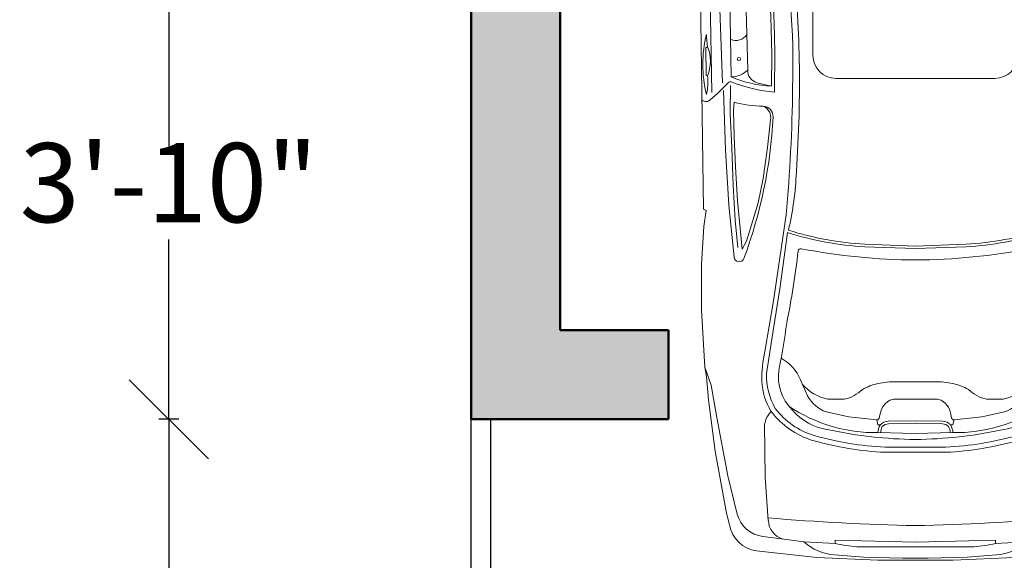
# Model space of a CAD drawing. Units: inches. Extents: x 3121 to 3511, y 1323 to 1998.
# Tile 2 of 10: x 3144 to 3244, y 1402 to 1456. Entities that reach past the tile are written whole.
import ezdxf

# ---------------------------------------------------------------- set-up
doc = ezdxf.new("R2010")
doc.units = ezdxf.units.IN
for name, color, linetype, lineweight in [('0_Equip', 250, 'Continuous', 13), ('A-ANNO-DIMS', 2, 'Continuous', 18), ('A-FLOR', 7, 'Continuous', 25), ('A-WALL', 7, 'Continuous', 50), ('A-WALL-PATT', 3, 'Continuous', 13)]:
    doc.layers.add(name, color=color, linetype=linetype, lineweight=lineweight)
doc.styles.get("Standard").update_dxf_attribs({"font": 'arial.ttf'})
doc.dimstyles.new('ISO-25', dxfattribs={"dimtxt": 8, "dimasz": 8, "dimexe": 1, "dimexo": 1, "dimtad": 0, "dimtih": 1, "dimtoh": 1, "dimlunit": 3, "dimtxsty": 'Standard', "dimblk": 'OBLIQUE', "dimcen": 2.5, "dimclrt": 1, "dimadec": 0, "dimazin": 0, "dimtfac": 1, "dimtmove": 0, "dimatfit": 3, "dimfxl": 1, "dimfxlon": 1, "dimarcsym": 0})

# ---------------------------------------------------------------- blocks, each defined once
blk = doc.blocks.new('A$C4C7B54D1')
at = {"layer": '0_Equip', "ltscale": 0.1}
for p, q in [((-0.7257, 2.678), (-0.8531, 2.6707)), ((-0.7257, 2.678), (-0.5983, 2.6707)), ((-1.112, 2.6343), (-1.2037, 2.6168)), ((-1.0138, 2.6343), (-1.1673, 2.6045)), ((-1.0176, 2.6505), (-1.112, 2.6343)), ((-0.8531, 2.6707), (-1.0176, 2.6505)), ((-0.5983, 2.6707), (-0.4338, 2.6505)), ((-0.4376, 2.6343), (-0.284, 2.6045)), ((-0.4338, 2.6505), (-0.3394, 2.6343)), ((-0.3394, 2.6343), (-0.2477, 2.6168)), ((-1.2037, 2.6168), (-1.3142, 2.5898)), ((-1.1673, 2.6045), (-1.2824, 2.5829)), ((-0.8877, 2.6027), (-0.9812, 2.5937)), ((-0.8072, 2.6112), (-0.8877, 2.6027)), ((-0.7257, 2.6157), (-0.8072, 2.6112)), ((-0.7257, 2.6157), (-0.6441, 2.6112)), ((-0.6441, 2.6112), (-0.5636, 2.6027)), ((-0.5636, 2.6027), (-0.4701, 2.5937)), ((-0.284, 2.6045), (-0.1689, 2.5829)), ((-0.2477, 2.6168), (-0.1371, 2.5898)), ((-1.4032, 2.5628), (-1.4801, 2.5318)), ((-1.3789, 2.557), (-1.4667, 2.5181)), ((-1.3142, 2.5898), (-1.4032, 2.5628)), ((-1.2824, 2.5829), (-1.3789, 2.557)), ((-0.1689, 2.5829), (-0.0725, 2.557)), ((-0.1371, 2.5898), (-0.0481, 2.5628)), ((-0.0725, 2.557), (0.0153, 2.5181)), ((-0.0481, 2.5628), (0.0288, 2.5318)), ((-1.4667, 2.5181), (-1.5113, 2.4907)), ((0.0153, 2.5181), (0.06, 2.4907)), ((-1.5113, 2.4907), (-1.5393, 2.4562)), ((-1.1083, 2.5037), (-1.1486, 2.3827)), ((-0.343, 2.5037), (-0.3027, 2.3827)), ((0.06, 2.4907), (0.0879, 2.4562)), ((-1.5353, 2.3701), (-1.5529, 2.308)), ((-1.435, 2.1869), (-1.4221, 2.3511)), ((-1.1486, 2.3827), (-1.1961, 2.1797)), ((-0.3027, 2.3827), (-0.2552, 2.1797)), ((-0.0163, 2.1869), (-0.0293, 2.3511)), ((0.084, 2.3701), (0.1016, 2.308)), ((-1.5529, 2.308), (-1.5677, 2.2486)), ((0.1016, 2.308), (0.1164, 2.2486)), ((-1.5677, 2.2486), (-1.5849, 2.1795)), ((0.1164, 2.2486), (0.1336, 2.1795)), ((-1.597, 2.1976), (-1.615, 2.1169)), ((-1.6012, 2.2082), (-1.597, 2.1976)), ((-1.4537, 1.863), (-1.435, 2.1869)), ((0.0024, 1.863), (-0.0163, 2.1869)), ((0.1499, 2.2082), (0.1457, 2.1976)), ((0.1457, 2.1976), (0.1637, 2.1169)), ((-1.5849, 2.1795), (-1.5997, 2.1304)), ((-1.1961, 2.1797), (-1.2349, 1.9911)), ((-0.2552, 2.1797), (-0.2164, 1.9911)), ((0.1336, 2.1795), (0.1484, 2.1304)), ((-1.615, 2.1169), (-1.6235, 1.8165)), ((-1.5997, 2.1304), (-1.6161, 2.0798)), ((0.1484, 2.1304), (0.1647, 2.0798)), ((0.1637, 2.1169), (0.1722, 1.8165)), ((-1.2349, 1.9911), (-1.2767, 1.8097)), ((-0.2164, 1.9911), (-0.1746, 1.8097)), ((-1.566, 1.8774), (-1.5761, 1.5304)), ((-1.4681, 1.48), (-1.4537, 1.863)), ((0.0168, 1.48), (0.0024, 1.863)), ((0.1147, 1.8774), (0.1247, 1.5304)), ((-1.6235, 1.8165), (-1.6256, 1.5098)), ((-1.2767, 1.8097), (-1.3098, 1.588)), ((-0.1746, 1.8097), (-0.1415, 1.588)), ((0.1722, 1.8165), (0.1743, 1.5098)), ((-1.3098, 1.588), (-1.3443, 1.3187)), ((-0.1415, 1.588), (-0.107, 1.3187)), ((-1.6256, 1.5098), (-1.6129, 1.3846)), ((-1.5761, 1.5304), (-1.5789, 1.1834)), ((0.1247, 1.5304), (0.1276, 1.1834)), ((0.1743, 1.5098), (0.1616, 1.3846)), ((-1.461, 1.1868), (-1.4681, 1.48)), ((-0.955, 1.4459), (-0.955, 1.4827)), ((-0.955, 1.4827), (-0.9321, 1.4827)), ((-0.9321, 1.4827), (-0.9321, 1.4459)), ((-0.5192, 1.4827), (-0.5192, 1.4459)), ((-0.4964, 1.4827), (-0.5192, 1.4827)), ((-0.4964, 1.4459), (-0.4964, 1.4827)), ((0.0097, 1.1868), (0.0168, 1.48)), ((-0.9321, 1.4459), (-0.955, 1.4459)), ((-0.8614, 1.4242), (-0.8603, 1.382)), ((-0.6135, 1.4258), (-0.6012, 1.3814)), ((-0.5809, 1.3459), (-0.5793, 1.4233)), ((-0.5192, 1.4459), (-0.4964, 1.4459)), ((-1.6193, 1.3782), (-1.6252, 0.9375)), ((-1.6129, 1.3846), (-1.6193, 1.3782)), ((-0.8878, 1.3764), (-1.0456, 1.313)), ((-0.7861, 1.3973), (-0.8878, 1.3764)), ((0.1616, 1.3846), (0.1679, 1.3782)), ((0.1679, 1.3782), (0.1739, 0.9375)), ((-0.8835, 1.3269), (-0.7975, 1.3408)), ((-1.0456, 1.313), (-1.4462, 1.1776)), ((-1.0263, 1.2883), (-0.9361, 1.3119)), ((-0.9361, 1.3119), (-0.8835, 1.3269)), ((-1.2207, 1.2292), (-1.0263, 1.2883)), ((-1.4366, 1.1604), (-1.2207, 1.2292)), ((-1.3162, 1.2215), (-1.3088, 1.2011)), ((-1.0667, 1.22), (-1.1723, 1.1976)), ((-0.3847, 1.22), (-0.279, 1.1976)), ((-1.4565, 1.1447), (-1.461, 1.1868)), ((-1.4462, 1.1776), (-1.4366, 1.1604)), ((-1.1723, 1.1976), (-1.2762, 1.1716)), ((-0.7257, 1.1776), (-0.8858, 1.1725)), ((-0.7257, 1.1776), (-0.5655, 1.1725)), ((-0.279, 1.1976), (-0.1751, 1.1716)), ((0.0052, 1.1447), (0.0097, 1.1868)), ((-1.5793, 1.1562), (-1.5793, 0.9761)), ((-1.5552, 1.139), (-1.5552, 0.9693)), ((-1.4503, 1.1151), (-1.4565, 1.1447)), ((-1.3515, 1.142), (-1.3703, 1.1286)), ((-1.2762, 1.1716), (-1.3515, 1.142)), ((-0.1751, 1.1716), (-0.0999, 1.142)), ((-0.0999, 1.142), (-0.0811, 1.1286)), ((-0.0011, 1.1151), (0.0052, 1.1447)), ((0.1038, 1.139), (0.1038, 0.9693)), ((0.128, 1.1562), (0.128, 0.9761)), ((-1.444, 1.0892), (-1.4503, 1.1151)), ((-1.39, 1.0981), (-1.3927, 1.0739)), ((-1.3828, 1.1133), (-1.39, 1.0981)), ((-1.3703, 1.1286), (-1.3828, 1.1133)), ((-0.0811, 1.1286), (-0.0685, 1.1133)), ((-0.0685, 1.1133), (-0.0614, 1.0981)), ((-0.0614, 1.0981), (-0.0587, 1.0739)), ((-0.0073, 1.0892), (-0.0011, 1.1151)), ((-1.4368, 1.0623), (-1.444, 1.0892)), ((-1.4243, 1.0229), (-1.4368, 1.0623)), ((-1.3927, 1.0739), (-1.3918, 1.0533)), ((-1.3918, 1.0533), (-1.3867, 1.0211)), ((-0.0596, 1.0533), (-0.0646, 1.0211)), ((-0.0587, 1.0739), (-0.0596, 1.0533)), ((-0.027, 1.0229), (-0.0145, 1.0623)), ((-0.0145, 1.0623), (-0.0073, 1.0892)), ((-1.4064, 0.961), (-1.4243, 1.0229)), ((-1.3867, 1.0211), (-1.3374, 0.8446)), ((-0.0646, 1.0211), (-0.1139, 0.8446)), ((-0.0449, 0.961), (-0.027, 1.0229)), ((-1.5149, 1.011), (-1.4844, 0.9277)), ((0.0635, 1.011), (0.0331, 0.9277)), ((-1.6252, 0.9375), (-1.6745, 0.908)), ((-1.6252, 0.9375), (-1.5546, 0.9696)), ((-1.3759, 0.8562), (-1.4064, 0.961)), ((-0.0754, 0.8562), (-0.0449, 0.961)), ((0.1739, 0.9375), (0.1032, 0.9696)), ((0.1739, 0.9375), (0.2232, 0.908)), ((-1.6745, 0.908), (-1.7088, 0.8764)), ((-1.508, 0.8914), (-1.5321, 0.8786)), ((-1.4844, 0.9277), (-1.4486, 0.8345)), ((0.0331, 0.9277), (-0.0028, 0.8345)), ((0.0566, 0.8914), (0.0807, 0.8786)), ((0.2232, 0.908), (0.2574, 0.8764)), ((-1.5321, 0.8786), (-1.7381, 0.7945)), ((-1.5253, 0.865), (-1.7329, 0.7802)), ((-1.7088, 0.8764), (-1.728, 0.8432)), ((-1.5273, 0.8512), (-1.7203, 0.7738)), ((-1.4835, -0.0735), (-1.497, 0.863)), ((-1.3401, 0.7406), (-1.3759, 0.8562)), ((-0.1112, 0.7406), (-0.0754, 0.8562)), ((0.0322, -0.0735), (0.0457, 0.863)), ((0.074, 0.865), (0.2816, 0.7802)), ((0.0759, 0.8512), (0.269, 0.7738)), ((0.0807, 0.8786), (0.2867, 0.7945)), ((0.2574, 0.8764), (0.2767, 0.8432)), ((-1.7366, 0.8127), (-1.7377, 0.7934)), ((-1.728, 0.8432), (-1.7366, 0.8127)), ((-1.6171, 0.8152), (-1.5964, -0.6171)), ((-1.5805, 0.8299), (-1.5623, -0.138)), ((-1.5337, 0.8406), (-1.5355, 0.484)), ((-1.4486, 0.8345), (-1.4226, 0.7503)), ((-1.3374, 0.8446), (-1.3097, 0.7577)), ((-0.1139, 0.8446), (-0.1417, 0.7577)), ((-0.0028, 0.8345), (-0.0287, 0.7503)), ((0.0824, 0.8406), (0.0842, 0.484)), ((0.1292, 0.8299), (0.111, -0.138)), ((0.1658, 0.8152), (0.145, -0.6171)), ((0.2767, 0.8432), (0.2853, 0.8127)), ((0.2853, 0.8127), (0.2863, 0.7934)), ((-1.7377, 0.7934), (-1.7327, 0.7794)), ((-1.4352, 0.792), (-1.4152, -0.045)), ((-0.0162, 0.792), (-0.0361, -0.045)), ((0.2863, 0.7934), (0.2813, 0.7794)), ((-1.4226, 0.7503), (-1.4029, 0.6849)), ((-1.315, 0.66), (-1.3401, 0.7406)), ((-1.3097, 0.7577), (-1.2953, 0.7129)), ((-0.7926, 0.7532), (-0.8418, 0.7514)), ((-0.7257, 0.7541), (-0.7926, 0.7532)), ((-0.7257, 0.7541), (-0.6587, 0.7532)), ((-0.6587, 0.7532), (-0.6095, 0.7514)), ((-0.1417, 0.7577), (-0.156, 0.7129)), ((-0.1363, 0.66), (-0.1112, 0.7406)), ((-0.0287, 0.7503), (-0.0484, 0.6849)), ((-1.2953, 0.7129), (-1.2801, 0.6573)), ((-0.156, 0.7129), (-0.1712, 0.6573)), ((-1.4029, 0.6849), (-1.368, 0.5729)), ((-1.2951, 0.5849), (-1.315, 0.66)), ((-1.2801, 0.6573), (-1.2795, 0.6546)), ((-0.9389, 0.6526), (-1.0437, 0.6403)), ((-0.8346, 0.6593), (-0.9389, 0.6526)), ((-0.7257, 0.6582), (-0.8346, 0.6593)), ((-0.7257, 0.6582), (-0.6168, 0.6593)), ((-0.6168, 0.6593), (-0.5124, 0.6526)), ((-0.5124, 0.6526), (-0.4076, 0.6403)), ((-0.1712, 0.6573), (-0.1719, 0.6546)), ((-0.1562, 0.5849), (-0.1363, 0.66)), ((-0.0484, 0.6849), (-0.0834, 0.5729)), ((-1.2021, 0.6133), (-1.2663, 0.5956)), ((-1.1177, 0.6302), (-1.2021, 0.6133)), ((-1.1142, 0.6096), (-1.1973, 0.593)), ((-1.0437, 0.6403), (-1.1177, 0.6302)), ((-1.0411, 0.6196), (-1.1142, 0.6096)), ((-0.937, 0.6317), (-1.0411, 0.6196)), ((-0.834, 0.6384), (-0.937, 0.6317)), ((-0.7257, 0.6373), (-0.834, 0.6384)), ((-0.7257, 0.6373), (-0.6173, 0.6384)), ((-0.6173, 0.6384), (-0.5143, 0.6317)), ((-0.5143, 0.6317), (-0.4102, 0.6196)), ((-0.4102, 0.6196), (-0.3371, 0.6096)), ((-0.4076, 0.6403), (-0.3337, 0.6302)), ((-0.3371, 0.6096), (-0.2541, 0.593)), ((-0.3337, 0.6302), (-0.2492, 0.6133)), ((-0.2492, 0.6133), (-0.185, 0.5956)), ((-1.368, 0.5729), (-1.3527, 0.5066)), ((-1.2663, 0.5956), (-1.2951, 0.5849)), ((-1.2879, 0.5653), (-1.2951, 0.5849)), ((-1.2599, 0.5757), (-1.2879, 0.5653)), ((-1.1973, 0.593), (-1.2599, 0.5757)), ((-0.2541, 0.593), (-0.1914, 0.5757)), ((-0.1914, 0.5757), (-0.1635, 0.5653)), ((-0.185, 0.5956), (-0.1562, 0.5849)), ((-0.1635, 0.5653), (-0.1562, 0.5849)), ((-0.0834, 0.5729), (-0.0986, 0.5066)), ((-1.3527, 0.5066), (-1.3411, 0.4394)), ((-0.0986, 0.5066), (-0.1102, 0.4394)), ((-1.5355, 0.484), (-1.5292, 0.2045)), ((0.0842, 0.484), (0.0779, 0.2045)), ((-1.3411, 0.4394), (-1.3321, 0.3749)), ((-0.7257, 0.4085), (-1.0528, 0.4085)), ((-0.7257, 0.4085), (-0.3986, 0.4085)), ((-0.1102, 0.4394), (-0.1192, 0.3749)), ((-1.3321, 0.3749), (-1.3286, 0.3301)), ((-0.1192, 0.3749), (-0.1228, 0.3301)), ((-1.3286, 0.3301), (-1.3204, 0.1751)), ((-1.3178, 0.3418), (-1.31, 0.2426)), ((-0.1335, 0.3418), (-0.1413, 0.2426)), ((-0.1228, 0.3301), (-0.1309, 0.1751)), ((-1.1468, 0.3145), (-1.1468, 0.0145)), ((-0.3045, 0.3145), (-0.3045, 0.0145)), ((-1.5292, 0.2045), (-1.5185, -0.0974)), ((-1.31, 0.2426), (-1.306, 0.1454)), ((-0.1413, 0.2426), (-0.1454, 0.1454)), ((0.0779, 0.2045), (0.0672, -0.0974)), ((-1.3204, 0.1751), (-1.3164, 0.0193)), ((-0.1309, 0.1751), (-0.1349, 0.0193)), ((-1.306, 0.1454), (-1.3036, 0.0305)), ((-0.1454, 0.1454), (-0.1478, 0.0305)), ((-1.5798, 0.0505), (-1.5879, 0.0456)), ((-1.5879, 0.0456), (-1.5863, -0.0676)), ((0.1285, 0.0505), (0.1365, 0.0456)), ((0.1365, 0.0456), (0.1349, -0.0676)), ((-1.3164, 0.0193), (-1.3178, -0.1112)), ((-1.3036, 0.0305), (-1.3044, -0.1358)), ((-0.1478, 0.0305), (-0.147, -0.1358)), ((-0.1349, 0.0193), (-0.1335, -0.1112)), ((-1.5863, -0.0676), (-1.5806, -0.0692)), ((-0.7257, -0.0796), (-1.0528, -0.0796)), ((-0.7257, -0.0796), (-0.3986, -0.0796)), ((0.1349, -0.0676), (0.1293, -0.0692)), ((-1.4948, -0.0965), (-1.5413, -0.143)), ((-1.4857, -0.1082), (-1.4866, -0.2223)), ((-1.3774, -0.0972), (-1.3178, -0.1112)), ((-0.0739, -0.0972), (-0.1335, -0.1112)), ((0.0344, -0.1082), (0.0352, -0.2223)), ((0.0435, -0.0965), (0.0899, -0.143)), ((-1.5413, -0.143), (-1.5686, -0.1663)), ((-1.5147, -0.1299), (-1.5058, -0.3725)), ((0.0633, -0.1299), (0.0545, -0.3725)), ((0.0899, -0.143), (0.1172, -0.1663)), ((-1.4713, -0.1773), (-1.4737, -0.2127)), ((0.02, -0.1773), (0.0224, -0.2127)), ((-1.4866, -0.2223), (-1.4809, -0.3653)), ((-1.4737, -0.2127), (-1.4705, -0.3187)), ((0.0224, -0.2127), (0.0192, -0.3187)), ((0.0352, -0.2223), (0.0296, -0.3653)), ((-1.3211, -0.2496), (-1.3332, -0.3629)), ((-0.1302, -0.2496), (-0.1182, -0.3629)), ((-1.4705, -0.3187), (-1.4649, -0.4424)), ((0.0192, -0.3187), (0.0135, -0.4424)), ((-1.3332, -0.3629), (-1.3516, -0.4906)), ((-0.1182, -0.3629), (-0.0997, -0.4906)), ((-1.5058, -0.3725), (-1.4922, -0.6007)), ((-1.4809, -0.3653), (-1.4745, -0.5203)), ((0.0296, -0.3653), (0.0232, -0.5203)), ((0.0545, -0.3725), (0.0408, -0.6007)), ((-1.4649, -0.4424), (-1.4576, -0.5822)), ((0.0135, -0.4424), (0.0063, -0.5822)), ((-1.4745, -0.5203), (-1.4665, -0.6617)), ((-1.3516, -0.4906), (-1.3725, -0.5902)), ((-0.0997, -0.4906), (-0.0788, -0.5902)), ((0.0232, -0.5203), (0.0151, -0.6617)), ((-1.4922, -0.6007), (-1.4712, -0.814)), ((-1.4576, -0.5822), (-1.4384, -0.7806)), ((-1.3725, -0.5902), (-1.3942, -0.6641)), ((-0.0788, -0.5902), (-0.0571, -0.6641)), ((0.0063, -0.5822), (-0.013, -0.7806)), ((0.0408, -0.6007), (0.0198, -0.814)), ((-1.5964, -0.6171), (-1.5863, -0.6228)), ((-1.5863, -0.6228), (-1.5949, -0.6885)), ((-1.3094, -0.9936), (-1.2569, -0.6398)), ((-0.1419, -0.9936), (-0.1944, -0.6398)), ((0.145, -0.6171), (0.1349, -0.6228)), ((0.1349, -0.6228), (0.1436, -0.6885)), ((-1.4665, -0.6617), (-1.4552, -0.7742)), ((-1.3942, -0.6641), (-1.4199, -0.7485)), ((-0.0571, -0.6641), (-0.0314, -0.7485)), ((0.0151, -0.6617), (0.0039, -0.7742)), ((-1.5949, -0.6885), (-1.605, -0.843)), ((-1.2616, -0.7846), (-1.2511, -0.7134)), ((-0.1898, -0.7846), (-0.2003, -0.7134)), ((0.1436, -0.6885), (0.1537, -0.843)), ((-1.4199, -0.7485), (-1.4384, -0.7806)), ((-0.9331, -0.7613), (-0.7253, -0.7683)), ((-0.5182, -0.7613), (-0.726, -0.7683)), ((-0.0314, -0.7485), (-0.013, -0.7806)), ((-1.2826, -0.9445), (-1.2616, -0.7846)), ((-0.9336, -0.7717), (-0.7257, -0.7787)), ((-0.5177, -0.7717), (-0.7257, -0.7787)), ((-0.1688, -0.9445), (-0.1898, -0.7846)), ((-1.605, -0.843), (-1.605, -1.0322)), ((0.1537, -0.843), (0.1537, -1.0322)), ((-1.3094, -1.1068), (-1.2826, -0.9445)), ((-0.1419, -1.1068), (-0.1688, -0.9445)), ((-1.3444, -1.2014), (-1.3094, -0.9936)), ((-0.1069, -1.2014), (-0.1419, -0.9936)), ((-1.605, -1.0322), (-1.592, -1.2661)), ((0.1537, -1.0322), (0.1407, -1.2661)), ((-1.3386, -1.2925), (-1.3094, -1.1068)), ((-0.1127, -1.2925), (-0.1419, -1.1068)), ((-1.565, -1.3405), (-1.592, -1.2661)), ((-1.592, -1.2661), (-1.5848, -1.3051)), ((0.1137, -1.3405), (0.1407, -1.2661)), ((0.1407, -1.2661), (0.1335, -1.3051)), ((-1.5848, -1.3051), (-1.5762, -1.4004)), ((-1.1985, -1.3182), (-1.1694, -1.3835)), ((-0.88, -1.3337), (-0.8328, -1.3271)), ((-0.8328, -1.3271), (-0.7257, -1.3271)), ((-0.6185, -1.3271), (-0.7257, -1.3271)), ((-0.5713, -1.3337), (-0.6185, -1.3271)), ((-0.2528, -1.3182), (-0.282, -1.3835)), ((0.1335, -1.3051), (0.1248, -1.4004)), ((-1.5417, -1.4736), (-1.565, -1.3405)), ((0.0904, -1.4736), (0.1137, -1.3405)), ((-1.5762, -1.4004), (-1.5486, -1.6107)), ((-1.0858, -1.3979), (-1.0181, -1.3979)), ((-0.8488, -1.4158), (-0.8558, -1.4236)), ((-0.8409, -1.4088), (-0.8488, -1.4158)), ((-0.8309, -1.402), (-0.8409, -1.4088)), ((-0.8163, -1.3979), (-0.8309, -1.402)), ((-0.7257, -1.3974), (-0.8163, -1.3979)), ((-0.7257, -1.3974), (-0.635, -1.3979)), ((-0.635, -1.3979), (-0.6204, -1.402)), ((-0.6204, -1.402), (-0.6104, -1.4088)), ((-0.6104, -1.4088), (-0.6025, -1.4158)), ((-0.6025, -1.4158), (-0.5955, -1.4236)), ((-0.3655, -1.3979), (-0.4333, -1.3979)), ((0.1248, -1.4004), (0.0973, -1.6107)), ((-1.0923, -1.4501), (-0.9989, -1.4699)), ((-0.8696, -1.4545), (-0.8731, -1.467)), ((-0.8664, -1.4423), (-0.8696, -1.4545)), ((-0.861, -1.4312), (-0.8664, -1.4423)), ((-0.8558, -1.4236), (-0.861, -1.4312)), ((-0.5955, -1.4236), (-0.5904, -1.4312)), ((-0.5904, -1.4312), (-0.585, -1.4423)), ((-0.585, -1.4423), (-0.5817, -1.4545)), ((-0.5817, -1.4545), (-0.5782, -1.467)), ((-0.359, -1.4501), (-0.4524, -1.4699)), ((-1.4962, -1.7129), (-1.5417, -1.4736)), ((-0.9989, -1.4699), (-0.8846, -1.4828)), ((-0.8807, -1.4821), (-0.8846, -1.4828)), ((-0.8846, -1.4828), (-0.8799, -1.5038)), ((-0.8769, -1.4791), (-0.8807, -1.4821)), ((-0.8745, -1.477), (-0.8769, -1.4791)), ((-0.8731, -1.467), (-0.8745, -1.477)), ((-0.7257, -1.4865), (-0.8374, -1.4884)), ((-0.7257, -1.4969), (-0.837, -1.4988)), ((-0.7257, -1.4865), (-0.6139, -1.4884)), ((-0.7257, -1.4969), (-0.6143, -1.4988)), ((-0.5782, -1.467), (-0.5768, -1.477)), ((-0.5768, -1.477), (-0.5744, -1.4791)), ((-0.5744, -1.4791), (-0.5706, -1.4821)), ((-0.5668, -1.4828), (-0.5714, -1.5038)), ((-0.5706, -1.4821), (-0.5668, -1.4828)), ((-0.4524, -1.4699), (-0.5668, -1.4828)), ((0.0448, -1.7129), (0.0904, -1.4736)), ((-1.3456, -1.5004), (-1.3433, -1.7188)), ((-0.8799, -1.5038), (-0.8706, -1.5038)), ((-0.8799, -1.5352), (-0.7257, -1.5393)), ((-0.5714, -1.5352), (-0.7257, -1.5393)), ((-0.5714, -1.5038), (-0.5808, -1.5038)), ((-0.1057, -1.5004), (-0.1081, -1.7188)), ((-1.5486, -1.6107), (-1.5024, -1.8663)), ((-0.8507, -1.616), (-0.7257, -1.616)), ((-0.8502, -1.5951), (-0.7257, -1.5951)), ((-0.6011, -1.5951), (-0.7257, -1.5951)), ((-0.6006, -1.616), (-0.7257, -1.616)), ((0.0973, -1.6107), (0.0511, -1.8663)), ((-1.4584, -1.8701), (-1.4962, -1.7129)), ((-1.3433, -1.7188), (-1.3304, -1.8962)), ((-0.1081, -1.7188), (-0.1209, -1.8962)), ((0.0071, -1.8701), (0.0448, -1.7129)), ((-1.5024, -1.8663), (-1.4894, -1.914)), ((0.0511, -1.8663), (0.0381, -1.914)), ((-1.2767, -1.9721), (-1.3526, -1.9616)), ((-1.1845, -1.9838), (-1.2767, -1.9721)), ((-1.055, -1.9768), (-1.055, -1.9908)), ((-0.7257, -1.985), (-1.055, -1.9768)), ((-0.7257, -1.985), (-0.3964, -1.9768)), ((-0.3964, -1.9768), (-0.3964, -1.9908)), ((-0.2668, -1.9838), (-0.1746, -1.9721)), ((-0.1746, -1.9721), (-0.0987, -1.9616)), ((-1.3797, -2.0208), (-1.1314, -2.0483)), ((-1.055, -1.9908), (-1.1845, -1.9838)), ((-0.9663, -2.0048), (-0.7257, -2.0048)), ((-0.4851, -2.0048), (-0.7257, -2.0048)), ((-0.3964, -1.9908), (-0.2668, -1.9838)), ((-0.0716, -2.0208), (-0.3199, -2.0483)), ((-1.1314, -2.0483), (-0.8803, -2.0598)), ((-1.0585, -2.0375), (-0.9383, -2.0469)), ((-0.9383, -2.0469), (-0.7784, -2.0504)), ((-0.8803, -2.0598), (-0.7257, -2.0598)), ((-0.7784, -2.0504), (-0.7257, -2.0504)), ((-0.673, -2.0504), (-0.7257, -2.0504)), ((-0.5711, -2.0598), (-0.7257, -2.0598)), ((-0.5131, -2.0469), (-0.673, -2.0504)), ((-0.3199, -2.0483), (-0.5711, -2.0598)), ((-0.3929, -2.0375), (-0.5131, -2.0469))]:
    blk.add_line(p, q, dxfattribs=at)
at = {"layer": '0_Equip'}
for p, q in [((-0.7257, 2.5926), (-0.7905, 2.5897)), ((-0.733, 2.5923), (-0.733, 2.5325)), ((-0.7257, 2.5926), (-0.6608, 2.5897)), ((-0.7183, 2.5923), (-0.7183, 2.5325)), ((-1.0577, 2.5343), (-0.8949, 2.5537)), ((-1.0475, 2.557), (-1.0545, 2.5425)), ((-1.0517, 2.5482), (-0.8949, 2.567)), ((-1.0364, 2.5634), (-1.0475, 2.557)), ((-0.9467, 2.5739), (-1.0364, 2.5634)), ((-0.8628, 2.5838), (-0.9467, 2.5739)), ((-0.8949, 2.567), (-0.8211, 2.5763)), ((-0.8949, 2.5537), (-0.8211, 2.5631)), ((-0.7905, 2.5897), (-0.8628, 2.5838)), ((-0.8211, 2.5763), (-0.738, 2.5791)), ((-0.8211, 2.5631), (-0.738, 2.5659)), ((-0.8211, 2.5498), (-0.738, 2.5526)), ((-0.738, 2.5791), (-0.733, 2.58)), ((-0.738, 2.5659), (-0.733, 2.5668)), ((-0.738, 2.5526), (-0.733, 2.5536)), ((-0.7133, 2.5791), (-0.7183, 2.58)), ((-0.7133, 2.5659), (-0.7183, 2.5668)), ((-0.7133, 2.5526), (-0.7183, 2.5536)), ((-0.6302, 2.5763), (-0.7133, 2.5791)), ((-0.6302, 2.5631), (-0.7133, 2.5659)), ((-0.6302, 2.5498), (-0.7133, 2.5526)), ((-0.6608, 2.5897), (-0.5886, 2.5838)), ((-0.5564, 2.567), (-0.6302, 2.5763)), ((-0.5564, 2.5537), (-0.6302, 2.5631)), ((-0.5886, 2.5838), (-0.5046, 2.5739)), ((-0.3996, 2.5482), (-0.5564, 2.567)), ((-0.3936, 2.5343), (-0.5564, 2.5537)), ((-0.5046, 2.5739), (-0.4149, 2.5634)), ((-0.4149, 2.5634), (-0.4038, 2.557)), ((-0.4038, 2.557), (-0.3968, 2.5425)), ((-1.0545, 2.5425), (-1.0638, 2.5185)), ((-1.0638, 2.5185), (-1.0638, 2.5092)), ((-1.0631, 2.5204), (-0.8949, 2.5405)), ((-1.0376, 2.5051), (-1.0067, 2.5116)), ((-1.0067, 2.5116), (-0.9502, 2.5168)), ((-0.9502, 2.5168), (-0.8657, 2.5238)), ((-0.8949, 2.5405), (-0.8211, 2.5498)), ((-0.8657, 2.5238), (-0.7922, 2.5308)), ((-0.7922, 2.5308), (-0.7433, 2.5325)), ((-0.7433, 2.5325), (-0.7257, 2.5325)), ((-0.7389, 2.5095), (-0.7395, 2.5059)), ((-0.708, 2.5325), (-0.7257, 2.5325)), ((-0.7124, 2.5095), (-0.7119, 2.5059)), ((-0.6591, 2.5308), (-0.708, 2.5325)), ((-0.5857, 2.5238), (-0.6591, 2.5308)), ((-0.5564, 2.5405), (-0.6302, 2.5498)), ((-0.5011, 2.5168), (-0.5857, 2.5238)), ((-0.3882, 2.5204), (-0.5564, 2.5405)), ((-0.4446, 2.5116), (-0.5011, 2.5168)), ((-0.4137, 2.5051), (-0.4446, 2.5116)), ((-0.3968, 2.5425), (-0.3875, 2.5185)), ((-0.3875, 2.5185), (-0.3875, 2.5092)), ((-1.0638, 2.5092), (-1.0545, 2.504)), ((-1.0545, 2.504), (-1.0376, 2.5051)), ((-0.7566, 2.4971), (-0.7261, 2.4828)), ((-0.7566, 2.4971), (-0.7291, 2.4776)), ((-0.7259, 2.4578), (-0.7291, 2.4776)), ((-0.6947, 2.4974), (-0.7261, 2.4828)), ((-0.7259, 2.4578), (-0.723, 2.4776)), ((-0.6947, 2.4974), (-0.723, 2.4776)), ((-0.3968, 2.504), (-0.4137, 2.5051)), ((-0.3875, 2.5092), (-0.3968, 2.504))]:
    blk.add_line(p, q, dxfattribs=at)
at = {"layer": '0_Equip', "ltscale": 0.1}
for centre in [(-1.4513, 0), (0, 0)]:
    blk.add_circle(centre, 0.00662, dxfattribs=at)
for centre, radius, start, end in [((-1.0252, 2.6508), 0.02, 304.7228, 3.5172), ((-0.4261, 2.6508), 0.02, 176.4828, 235.2772), ((-0.9299, 2.2354), 0.3619, 98.1466, 109.2524), ((-0.5214, 2.2354), 0.3619, 70.7476, 81.8534), ((-0.9799, 2.461), 0.1353, 120.8369, 151.2853), ((-0.4714, 2.461), 0.1353, 28.7147, 59.1631), ((-1.4391, 2.4422), 0.0986, 114.5945, 157.5113), ((-1.2153, 2.6098), 0.1432, 299.1564, 328.1831), ((-0.9799, 2.461), 0.1353, 151.2853, 161.5889), ((-1.0728, 2.5126), 0.029, 152.6038, 261.721), ((-0.6679, -0.6671), 3.1773, 91.0415, 97.3969), ((-0.7834, -0.6671), 3.1773, 82.6031, 88.9585), ((-0.3785, 2.5126), 0.029, 278.279, 27.3962), ((-0.236, 2.6098), 0.1432, 211.8169, 240.8436), ((-0.4714, 2.461), 0.1353, 18.4111, 28.7147), ((-0.0123, 2.4422), 0.0986, 22.4887, 65.4055), ((-0.4722, 2.0579), 1.139, 158.2564, 172.4203), ((-0.9791, 2.0579), 1.139, 7.5797, 21.7436), ((-1.4083, 2.3394), 0.1306, 130.2084, 166.4224), ((-1.4798, 2.4259), 0.0184, 54.8052, 134.0204), ((-1.2841, 2.5028), 0.0501, 260.5448, 306.7068), ((-0.1672, 2.5028), 0.0501, 233.2932, 279.4552), ((0.0285, 2.4259), 0.0184, 45.9796, 125.1948), ((-0.043, 2.3394), 0.1306, 13.5776, 49.7916), ((0.5502, 1.746), 1.9445, 161.1117, 170.7019), ((-2.0015, 1.746), 1.9445, 9.2981, 18.8883), ((1.1202, 1.7918), 2.6875, 169.5541, 178.1755), ((-2.5715, 1.7918), 2.6875, 1.8245, 10.4459), ((9.2655, 0.7813), 10.7109, 173.14258, 175.77374), ((-10.7169, 0.7813), 10.7109, 4.22626, 6.85742), ((2.9623, 1.2089), 4.3935, 175.2767, 179.1124), ((-4.4136, 1.2089), 4.3935, 0.8876, 4.7233), ((-0.7686, 0.201), 1.2267, 87.9955, 103.2364), ((-0.3726, 1.0935), 0.5131, 139.3585, 143.6922), ((-0.6528, 1.3354), 0.1211, 130.7679, 145.6911), ((-0.6828, 0.201), 1.2267, 76.7636, 92.0045), ((-0.786, 0.3109), 1.1158, 103.6551, 119.1148), ((-0.7554, 1.327), 0.0768, 88.1186, 113.6019), ((-0.7803, 1.3768), 0.0384, 357.9275, 44.3829), ((-0.6872, 1.4869), 0.1241, 243.8649, 311.6638), ((-0.6113, 1.3746), 0.0122, 294.8678, 33.6398), ((-0.6653, 0.3109), 1.1158, 60.8852, 76.3449), ((-0.9216, 1.3498), 0.0409, 323.4512, 39.0343), ((-0.8494, 1.486), 0.1542, 289.6676, 314.192), ((-0.7147, 1.4628), 0.1474, 235.8143, 265.7174), ((-0.741, 1.5272), 0.212, 274.1513, 309.4931), ((-0.617, 0.3882), 0.9584, 77.6919, 87.8428), ((-0.929, 0.5266), 0.803, 96.22, 121.6991), ((-0.5976, 0.2949), 1.0461, 55.3038, 79.8165), ((-1.1803, 0.9494), 0.3676, 113.8511, 139.7847), ((-0.2711, 0.9494), 0.3676, 40.2153, 66.1489), ((-0.7356, -0.4312), 1.6538, 89.6554, 111.9286), ((-0.7478, -0.378), 1.6295, 89.2231, 101.2856), ((-0.7036, -0.378), 1.6295, 78.7144, 90.7769), ((-0.7157, -0.4312), 1.6538, 68.0714, 90.3446), ((-1.6261, 1.102), 0.0813, 40.278, 87.0689), ((-1.2706, 1.0395), 0.2408, 142.2718, 177.7746), ((-0.7356, -0.4312), 1.6329, 89.6554, 111.9286), ((-0.7157, -0.4312), 1.6329, 68.0714, 90.3446), ((-0.1807, 1.0395), 0.2408, 2.2254, 37.7282), ((0.1747, 1.102), 0.0813, 92.9311, 139.722), ((-2.3477, 0.6968), 0.9076, 22.824, 30.2904), ((-0.85, 0.0855), 1.0875, 91.8892, 118.6013), ((-0.6014, 0.0855), 1.0875, 61.3987, 88.1108), ((0.8964, 0.6968), 0.9076, 149.7096, 157.176), ((-1.3493, 1.0932), 0.0105, 111.9286, 291.9286), ((-0.102, 1.0932), 0.0105, 248.0714, 68.0714), ((-1.4887, 1.0171), 0.0269, 132.3277, 193.1064), ((-6.6059, -0.8606), 5.4408, 15.0904, 20.5451), ((5.1546, -0.8606), 5.4408, 159.4549, 164.9096), ((0.0373, 1.0171), 0.0269, 346.8936, 47.6723), ((-1.5684, 0.9084), 0.0628, 344.3283, 77.2348), ((0.1171, 0.9084), 0.0628, 102.7652, 195.6717), ((-1.4233, 0.9849), 0.1262, 227.8287, 253.081), ((-0.0281, 0.9849), 0.1262, 286.919, 312.1713), ((-1.5495, 0.8614), 0.0245, 335.4987, 44.5114), ((-1.463, 0.9441), 0.0879, 224.7932, 273.9292), ((0.0117, 0.9441), 0.0879, 266.0708, 315.2068), ((0.0982, 0.8614), 0.0245, 135.4886, 204.5013), ((-1.7238, 0.7825), 0.00941, 199.646, 291.8616), ((0.2725, 0.7825), 0.00941, 248.1384, 340.354), ((-0.8474, 0.7163), 0.0355, 80.937, 162.15), ((-0.6039, 0.7163), 0.0355, 17.85, 99.063), ((-0.9515, 0.7495), 0.0737, 286.567, 342.4011), ((-0.4998, 0.7495), 0.0737, 197.5989, 253.433), ((-1.1535, 0.5061), 0.2334, 134.9877, 155.4049), ((-1.249, 0.662), 0.0314, 193.667, 283.2045), ((-0.7896, -1.2957), 1.9795, 94.0807, 103.2045), ((-0.6617, -1.2957), 1.9795, 76.7955, 85.9193), ((-0.2023, 0.662), 0.0314, 256.7955, 346.333), ((-0.2978, 0.5061), 0.2334, 24.5951, 45.0123), ((-2.0025, 0.3511), 0.7759, 4.7259, 16.8296), ((0.5512, 0.3511), 0.7759, 163.1704, 175.2741), ((-2.6334, 0.2371), 1.3197, 4.5498, 13.9797), ((-4.2099, -0.0242), 2.9809, 358.1905, 11.4064), ((2.7585, -0.0242), 2.9809, 168.5936, 181.8095), ((1.1821, 0.2371), 1.3197, 166.0203, 175.4502), ((-1.2324, 0.3484), 0.1397, 106.6168, 134.6647), ((-0.2189, 0.3484), 0.1397, 45.3353, 73.3832), ((-6.5594, -0.126), 5.3575, 1.3159, 5.7952), ((-1.0528, 0.3145), 0.0941, 90, 180), ((-0.3986, 0.3145), 0.0941, 0, 90), ((5.1081, -0.126), 5.3575, 174.2048, 178.6841), ((-1.0944, -0.0222), 0.5055, 165.8807, 194.1193), ((-1.3066, 0.102), 0.2781, 180.1936, 190.6834), ((-1.4634, 0.1296), 0.0534, 245.2796, 326.9469), ((0.0121, 0.1296), 0.0534, 213.0531, 294.7204), ((-0.1448, 0.102), 0.2781, 349.3166, 359.8064), ((-0.3569, -0.0222), 0.5055, 345.8807, 14.1193), ((-1.7275, -0.0084), 0.159, 337.4976, 21.7335), ((0.2762, -0.0084), 0.159, 158.2665, 202.5024), ((-1.0528, 0.0145), 0.0941, 180, 270), ((-0.3986, 0.0145), 0.0941, 270, 0), ((-6.573, -0.0941), 5.3705, 356.0501, 0.9723), ((5.1217, -0.0941), 5.3705, 179.0277, 183.9499), ((-1.7817, -0.0969), 0.2029, 346.1346, 7.8419), ((-1.4831, 0.0214), 0.095, 269.7172, 315.6185), ((-1.2968, 0.3651), 0.4767, 246.9385, 267.4714), ((-1.3634, -0.0473), 0.0519, 177.4537, 254.2676), ((-0.1545, 0.3651), 0.4767, 272.5286, 293.0615), ((-0.0879, -0.0473), 0.0519, 285.7324, 2.5463), ((0.0317, 0.0214), 0.095, 224.3815, 270.2828), ((0.3303, -0.0969), 0.2029, 172.1581, 193.8654), ((-1.4874, -0.1039), 0.0105, 68.8598, 135.0096), ((-1.2476, 0.5164), 0.6547, 248.8598, 265.0222), ((-8.0298, -0.0355), 6.7998, 354.90123, 359.30214), ((6.5785, -0.0355), 6.7998, 180.69786, 185.09877), ((-0.2038, 0.5164), 0.6547, 274.9778, 291.1402), ((0.0361, -0.1039), 0.0105, 44.9904, 111.1402), ((-1.5869, -0.1514), 0.0236, 227.2909, 320.7388), ((-1.3362, 0.3542), 0.5484, 255.7347, 268.4072), ((-1.3699, -0.2402), 0.0497, 349.0381, 68.1064), ((-1.3526, -0.2358), 0.0418, 357.143, 88.4072), ((-0.0988, -0.2358), 0.0418, 91.5928, 182.857), ((-0.0814, -0.2402), 0.0497, 111.8936, 190.9619), ((-0.1152, 0.3542), 0.5484, 271.5928, 284.2653), ((0.1355, -0.1514), 0.0236, 219.2612, 312.7091), ((-3.2483, -0.1412), 1.9399, 339.54, 357.143), ((1.797, -0.1412), 1.9399, 182.857, 200.46), ((-2.454, -0.4173), 1.2396, 346.6558, 357.8401), ((1.0027, -0.4173), 1.2396, 182.1599, 193.3442), ((-0.8588, 0.5276), 1.3014, 252.4566, 266.7043), ((-0.8588, 0.5276), 1.291, 252.4566, 266.6988), ((-0.5926, 0.5276), 1.291, 273.3012, 287.5434), ((-0.5926, 0.5276), 1.3014, 273.2957, 287.5434), ((-5.088, -0.3237), 3.9082, 348.7726, 353.1671), ((-1.1971, -0.7899), 0.0105, 79.1189, 173.1671), ((-0.7142, 1.7227), 2.5481, 259.1189, 269.7413), ((-0.7372, 1.7227), 2.5481, 270.2587, 280.8811), ((-0.2542, -0.7899), 0.0105, 6.8329, 100.8811), ((3.6366, -0.3237), 3.9082, 186.8329, 191.2274), ((-1.4504, -0.812), 0.0209, 185.6259, 339.54), ((-0.001, -0.812), 0.0209, 200.46, 354.3741), ((0.625, -1.1812), 0.5281, 165.7822, 187.813), ((0.1224, -1.0639), 0.0155, 11.61, 127.0083), ((-4.7286, -0.6026), 3.5073, 348.8701, 352.1003), ((3.2772, -0.6026), 3.5073, 187.8997, 191.1299), ((-0.7003, -1.1122), 0.8395, 350.5693, 3.5107), ((-0.8187, -1.3185), 0.5386, 167.4447, 180.7102), ((-0.6326, -1.3185), 0.5386, 359.2898, 12.5553), ((-1.3591, -1.3822), 0.1728, 21.7432, 61.9432), ((-0.0922, -1.3822), 0.1728, 118.0568, 158.2568), ((0.1138, -1.243), 0.0156, 219.7819, 334.4738), ((-1.0611, -1.2979), 0.2775, 178.8811, 209.7062), ((-1.0952, -1.3051), 0.1937, 172.4314, 224.4267), ((-0.3561, -1.3051), 0.1937, 315.5733, 7.5686), ((-0.3902, -1.2979), 0.2775, 330.2938, 1.1189), ((-1.0944, -1.3104), 0.2633, 183.2136, 211.504), ((-0.8301, -1.5634), 0.235, 102.268, 118.8572), ((-0.6213, -1.5634), 0.235, 61.1428, 77.732), ((-0.3569, -1.3104), 0.2633, 328.496, 356.7864), ((-1.0482, -1.2146), 0.1871, 220.4031, 258.3959), ((-1.0495, -1.2507), 0.1505, 282.0448, 314.7653), ((-0.4019, -1.2507), 0.1505, 225.2347, 257.9552), ((-0.4032, -1.2146), 0.1871, 281.6041, 319.5969), ((-1.0421, -1.3141), 0.145, 208.6187, 249.7318), ((-0.4092, -1.3141), 0.145, 290.2682, 331.3813), ((-1.2501, -1.516), 0.0967, 135.2951, 170.7274), ((-1.052, -1.2472), 0.3339, 216.9484, 253.2314), ((-1.052, -1.2472), 0.313, 216.9484, 253.2054), ((-0.8912, -0.9022), 0.6331, 235.8724, 271.0227), ((-1.0459, -1.2776), 0.2487, 221.0065, 261.6946), ((-0.5601, -0.9022), 0.6331, 268.9773, 304.1276), ((-0.4054, -1.2776), 0.2487, 278.3054, 318.9935), ((-0.3993, -1.2472), 0.313, 286.7946, 323.0516), ((-0.3993, -1.2472), 0.3339, 286.7686, 323.0516), ((-0.2012, -1.516), 0.0967, 9.2726, 44.7049), ((-0.8344, -1.538), 0.0498, 93.4455, 136.5439), ((-0.6169, -1.538), 0.0498, 43.4561, 86.5545), ((-0.7003, 0.2815), 1.8451, 258.0669, 269.2129), ((-0.8066, -1.54), 0.0735, 150.5285, 176.2825), ((-0.8066, -1.54), 0.063, 151.7195, 175.9212), ((-0.8344, -1.538), 0.0393, 93.7549, 134.7116), ((-0.751, 0.2815), 1.8451, 270.7871, 281.9331), ((-0.6169, -1.538), 0.0393, 45.2884, 86.2451), ((-0.6447, -1.54), 0.063, 4.0788, 28.2805), ((-0.6447, -1.54), 0.0735, 3.7175, 29.4715), ((-0.7884, -0.3101), 1.3074, 254.0198, 267.2681), ((-0.7884, -0.3101), 1.2865, 254.0263, 267.246), ((-0.6629, -0.3101), 1.2865, 272.754, 285.9737), ((-0.6629, -0.3101), 1.3074, 272.7319, 285.9802), ((-1.3393, -1.8393), 0.123, 194.4986, 263.7836), ((-0.5134, 7.9307), 9.8503, 265.23745, 268.76503), ((-1.2452, -1.8915), 0.0853, 183.2055, 252.6405), ((-0.938, 7.9307), 9.8503, 271.23497, 274.76255), ((-0.2061, -1.8915), 0.0853, 287.3595, 356.7945), ((-0.1121, -1.8393), 0.123, 276.2164, 345.5014), ((-1.3628, -1.8937), 0.1282, 189.093, 262.4153), ((-0.0885, -1.8937), 0.1282, 277.5847, 350.907), ((-1.0413, -1.8225), 0.2157, 228.406, 265.4391), ((-0.896, -1.272), 0.7362, 257.5275, 264.5209), ((-0.5554, -1.272), 0.7362, 275.4791, 282.4725), ((-0.41, -1.8225), 0.2157, 274.5609, 311.594)]:
    blk.add_arc(centre, radius, start, end, dxfattribs=at)
for centre, major_axis, ratio in [((-1.2016, 2.4892), (0.0562, 0.0189), 0.759763), ((-1.399, 2.4187), (-0.1036, -0.0518), 0.497493)]:
    blk.add_ellipse(centre, major_axis=major_axis, ratio=ratio, dxfattribs=at)
at = {"layer": '0_Equip', "ltscale": 0.1, "extrusion": (0, 0, -1)}
for centre, major_axis, ratio in [((-0.2497, 2.4892), (-0.0562, 0.0189), 0.759763), ((-0.0523, 2.4187), (0.1036, -0.0518), 0.497493)]:
    blk.add_ellipse(centre, major_axis=major_axis, ratio=ratio, dxfattribs=at)
at = {"layer": '0_Equip'}
blk.add_ellipse((-0.7253, 2.4812), major_axis=(-0.0426, 0), ratio=0.550187, dxfattribs=at)
at = {"layer": '0_Equip', "ltscale": 0.1}
for points, knots in [([(-1.1548, 2.5048), (-1.1596, 2.5191), (-1.1811, 2.5294), (-1.2283, 2.5198), (-1.248, 2.5001), (-1.2511, 2.4679), (-1.2373, 2.4539), (-1.1922, 2.4512), (-1.1656, 2.4658), (-1.1532, 2.4906), (-1.1526, 2.4983), (-1.1548, 2.5048)], [0, 0, 0, 0, 1.408119, 1.408119, 2.816238, 2.816238, 4.224358, 4.224358, 5.632477, 5.632477, 6.283185, 6.283185, 6.283185, 6.283185]), ([(-0.2965, 2.5048), (-0.2917, 2.5191), (-0.2703, 2.5294), (-0.2231, 2.5198), (-0.2033, 2.5001), (-0.2003, 2.4679), (-0.2141, 2.4539), (-0.2592, 2.4512), (-0.2858, 2.4658), (-0.2981, 2.4906), (-0.2987, 2.4983), (-0.2965, 2.5048)], [0, 0, 0, 0, 1.408119, 1.408119, 2.816238, 2.816238, 4.224358, 4.224358, 5.632477, 5.632477, 6.283185, 6.283185, 6.283185, 6.283185]), ([(-1.4937, 2.3714), (-1.4901, 2.3641), (-1.4809, 2.3581), (-1.4492, 2.3543), (-1.4277, 2.3571), (-1.3679, 2.3771), (-1.3298, 2.404), (-1.2994, 2.4483), (-1.2993, 2.4626), (-1.3171, 2.4801), (-1.3406, 2.4849), (-1.3989, 2.4733), (-1.4323, 2.4577), (-1.4816, 2.4186), (-1.4956, 2.3954), (-1.4959, 2.3774), (-1.4951, 2.3742), (-1.4937, 2.3714)], [0, 0, 0, 0, 0.646556, 0.646556, 1.293113, 1.293113, 2.410172, 2.410172, 3.309931, 3.309931, 4.20969, 4.20969, 5.109449, 5.109449, 6.031285, 6.031285, 6.283185, 6.283185, 6.283185, 6.283185]), ([(0.0424, 2.3714), (0.0388, 2.3641), (0.0295, 2.3581), (-0.0022, 2.3543), (-0.0236, 2.3571), (-0.0834, 2.3771), (-0.1216, 2.404), (-0.152, 2.4483), (-0.152, 2.4626), (-0.1343, 2.4801), (-0.1108, 2.4849), (-0.0524, 2.4733), (-0.019, 2.4577), (0.0303, 2.4186), (0.0443, 2.3954), (0.0445, 2.3774), (0.0438, 2.3742), (0.0424, 2.3714)], [0, 0, 0, 0, 0.646556, 0.646556, 1.293113, 1.293113, 2.410172, 2.410172, 3.309931, 3.309931, 4.20969, 4.20969, 5.109449, 5.109449, 6.031285, 6.031285, 6.283185, 6.283185, 6.283185, 6.283185])]:
    blk.add_open_spline(points, degree=3, knots=knots, dxfattribs=at)
at = {"layer": '0_Equip'}
blk.add_open_spline([(-0.7708, 2.4812), (-0.7708, 2.4725), (-0.7635, 2.4648), (-0.7294, 2.4499), (-0.6897, 2.4563), (-0.6733, 2.4916), (-0.7036, 2.5102), (-0.7526, 2.5051), (-0.7708, 2.4948), (-0.7708, 2.4812)], degree=3, knots=[0, 0, 0, 0, 0.903923, 0.903923, 2.878844, 2.878844, 4.872977, 4.872977, 6.283185, 6.283185, 6.283185, 6.283185], dxfattribs=at)
blk = doc.blocks.new('_Oblique')
at = {"color": 0, "linetype": 'ByBlock', "lineweight": -2}
blk.add_line((-0.5, -0.5), (0.5, 0.5), dxfattribs=at)
blk = doc.blocks.new('*D33')
at = {"layer": 'A-ANNO-DIMS', "color": 0, "lineweight": -2, "transparency": 16777216}
for p, q in [((3160.368, 1415.784), (3158.368, 1415.784)), ((3159.368, 1415.784), (3159.368, 1395.492)), ((3159.368, 1365.917), (3159.368, 1386.209)), ((3160.368, 1365.917), (3158.368, 1365.917))]:
    blk.add_line(p, q, dxfattribs=at)
at = {"layer": 'Defpoints', "color": 0, "transparency": 16777216}
for p in [(3159.368, 1415.784), (3189.918, 1415.784), (3189.918, 1365.917)]:
    blk.add_point(p, dxfattribs=at)
at = {"layer": 'A-ANNO-DIMS', "color": 0, "lineweight": -2, "transparency": 16777216, "xscale": 8, "yscale": 8, "zscale": 8}
for p, rotation in [((3159.368, 1415.784), 90), ((3159.368, 1365.917), 270)]:
    blk.add_blockref('_Oblique', p, dxfattribs=dict(at, rotation=rotation))
at = {"layer": 'A-ANNO-DIMS', "color": 1, "transparency": 16777216, "insert": (3159.368, 1390.851), "char_height": 8, "attachment_point": 5}
blk.add_mtext('4\'-2"', dxfattribs=at)
blk = doc.blocks.new('*D35')
at = {"layer": 'A-ANNO-DIMS', "color": 0, "lineweight": -2, "transparency": 16777216}
for p, q in [((3160.368, 1461.548), (3158.368, 1461.548)), ((3159.368, 1461.548), (3159.368, 1443.379)), ((3159.368, 1415.784), (3159.368, 1433.954)), ((3160.368, 1415.784), (3158.368, 1415.784))]:
    blk.add_line(p, q, dxfattribs=at)
at = {"layer": 'Defpoints', "color": 0, "transparency": 16777216}
for p in [(3159.368, 1461.548), (3189.918, 1461.548), (3189.918, 1415.784)]:
    blk.add_point(p, dxfattribs=at)
at = {"layer": 'A-ANNO-DIMS', "color": 0, "lineweight": -2, "transparency": 16777216, "xscale": 8, "yscale": 8, "zscale": 8}
for p, rotation in [((3159.368, 1461.548), 90), ((3159.368, 1415.784), 270)]:
    blk.add_blockref('_Oblique', p, dxfattribs=dict(at, rotation=rotation))
at = {"layer": 'A-ANNO-DIMS', "color": 1, "transparency": 16777216, "insert": (3159.368, 1438.666), "char_height": 8, "attachment_point": 5}
blk.add_mtext('3\'-10"', dxfattribs=at)
blk = doc.blocks.new('*D58')
at = {"layer": 'A-ANNO-DIMS', "color": 0, "lineweight": -2, "transparency": 16777216}
for p, q in [((3209.892, 1985.334), (3209.892, 1987.334)), ((3311.328, 1985.334), (3311.328, 1987.334)), ((3209.892, 1986.334), (3240.026, 1986.334)), ((3311.328, 1986.334), (3281.194, 1986.334))]:
    blk.add_line(p, q, dxfattribs=at)
at = {"layer": 'Defpoints', "color": 0, "transparency": 16777216}
for p in [(3311.328, 1986.334), (3209.892, 1424.784), (3311.328, 1424.784)]:
    blk.add_point(p, dxfattribs=at)
at = {"layer": 'A-ANNO-DIMS', "color": 0, "lineweight": -2, "transparency": 16777216, "xscale": 8, "yscale": 8, "zscale": 8, "rotation": 180}
blk.add_blockref('_Oblique', (3209.892, 1986.334), dxfattribs=at)
at = {"layer": 'A-ANNO-DIMS', "color": 0, "lineweight": -2, "transparency": 16777216, "xscale": 8, "yscale": 8, "zscale": 8}
blk.add_blockref('_Oblique', (3311.328, 1986.334), dxfattribs=at)
at = {"layer": 'A-ANNO-DIMS', "color": 1, "transparency": 16777216, "insert": (3260.61, 1986.334), "char_height": 8, "attachment_point": 5}
blk.add_mtext('8\'-5 1/2"', dxfattribs=at)

msp = doc.modelspace()

# ---------------------------------------------------------------- hatches: boundary and pattern name
at = {"layer": 'A-WALL-PATT'}
h = msp.add_hatch(color=256, dxfattribs=at)
h.dxf.hatch_style = 1
h.paths.add_polyline_path([(3274.023, 1955.784), (3189.918, 1955.784), (3189.918, 1910.219), (3198.918, 1910.219), (3198.918, 1946.784), (3259.023, 1946.784), (3259.023, 1921.61), (3261.023, 1921.61), (3261.023, 1946.784), (3274.023, 1946.784)])
h.paths.add_polyline_path([(3327.918, 1946.784), (3334.156, 1946.784), (3334.156, 1955.784), (3310.023, 1955.784), (3310.023, 1946.784), (3318.918, 1946.784), (3318.918, 1929.796), (3311.644, 1929.796), (3311.644, 1927.007), (3324.033, 1927.007), (3324.033, 1871.381), (3311.644, 1871.381), (3311.644, 1868.381), (3318.918, 1868.381), (3318.918, 1853.784), (3327.918, 1853.784)])
h.paths.add_polyline_path([(3456.918, 1955.784), (3384.562, 1955.784), (3384.562, 1946.784), (3447.918, 1946.784), (3447.918, 1877.779), (3456.918, 1877.779)])
h.paths.add_polyline_path([(3456.918, 1835.782), (3447.918, 1835.782), (3447.918, 1814.784), (3414.918, 1814.784), (3414.918, 1803.784), (3447.918, 1803.784), (3447.918, 1793.443), (3456.918, 1793.443)])
h.paths.add_polyline_path([(3456.918, 1558.434), (3447.918, 1558.434), (3447.918, 1547.784), (3375.918, 1547.784), (3375.918, 1598.784), (3378.918, 1598.784), (3378.918, 1602.284), (3375.918, 1602.284), (3375.918, 1674.284), (3369.918, 1674.284), (3369.918, 1547.784), (3364.418, 1547.784), (3364.418, 1538.784), (3447.918, 1538.784), (3447.918, 1512.628), (3456.918, 1512.628)])
h.paths.add_polyline_path([(3456.918, 1460.558), (3447.918, 1460.558), (3447.918, 1424.784), (3412.543, 1424.784), (3412.543, 1415.784), (3456.918, 1415.784)])
h.paths.add_polyline_path([(3358.149, 1424.784), (3322.918, 1424.784), (3322.918, 1538.784), (3328.418, 1538.784), (3328.418, 1547.784), (3308.208, 1547.784), (3308.208, 1538.784), (3318.918, 1538.784), (3318.918, 1424.784), (3311.328, 1424.784), (3311.328, 1415.784), (3358.149, 1415.784)])
h.paths.add_polyline_path([(3207.562, 1547.784), (3198.918, 1547.784), (3198.918, 1607.327), (3189.918, 1607.327), (3189.918, 1513.073), (3198.918, 1513.073), (3198.918, 1538.784), (3207.562, 1538.784)])
h.paths.add_polyline_path([(3198.918, 1461.548), (3189.918, 1461.548), (3189.918, 1415.784), (3209.892, 1415.784), (3209.892, 1424.784), (3198.918, 1424.784)])
h.paths.add_polyline_path([(3272.208, 1547.784), (3238.766, 1547.784), (3238.766, 1538.784), (3272.208, 1538.784)])
h.paths.add_polyline_path([(3261.023, 1748.784), (3198.918, 1748.784), (3198.918, 1768.387), (3189.918, 1768.387), (3189.918, 1692.279), (3198.918, 1692.279), (3198.918, 1739.784), (3261.023, 1739.784)])
h.paths.add_polyline_path([(3198.918, 1856.171), (3189.918, 1856.171), (3189.918, 1808.331), (3198.918, 1808.331), (3198.918, 1821.074), (3261.023, 1821.074), (3261.023, 1862.309), (3259.023, 1862.309), (3259.023, 1825.074), (3198.918, 1825.074)])

# ---------------------------------------------------------------- linework, layer by layer
at = {"layer": 'A-FLOR'}
for points in [[(3322.918, 1415.784), (3322.918, 1365.917), (3189.918, 1365.917), (3189.918, 1415.784)], [(3320.918, 1415.784), (3320.918, 1367.917), (3191.918, 1367.917), (3191.918, 1415.784)]]:
    msp.add_lwpolyline(points, dxfattribs=at)
at = {"layer": 'A-WALL'}
for p, q in [((3189.918, 1955.784), (3189.918, 1415.784)), ((3198.918, 1538.784), (3198.918, 1424.784)), ((3198.918, 1424.784), (3209.892, 1424.784)), ((3209.892, 1424.784), (3209.892, 1415.784)), ((3189.918, 1415.784), (3209.892, 1415.784))]:
    msp.add_line(p, q, dxfattribs=at)

# ---------------------------------------------------------------- block references
at = {"layer": '0_Equip', "xscale": 24.59625072819005, "yscale": 24.59625072819005, "zscale": 24.59625072819005}
msp.add_blockref('A$C4C7B54D1', (3252.699, 1452.199), dxfattribs=at)

# ---------------------------------------------------------------- dimensions: what is measured, and where the dimension line sits
at = {"layer": 'A-ANNO-DIMS'}
dim = msp.add_linear_dim(base=(3311.328, 1986.334), p1=(3209.892, 1424.784), p2=(3311.328, 1424.784), dimstyle='ISO-25', override={"dimdec": 1, "dimlfac": 1, "dimrnd": 0, "dimzin": 1, "dimdsep": 46, "dimlunit": 4, "dimfrac": 2}, dxfattribs=at)
dim.commit()
dim.dimension.update_dxf_attribs({"geometry": '*D58', "text_midpoint": (3260.61, 1986.334)})
for base, p1, p2, picture, middle in [((3159.368, 1461.548), (3189.918, 1415.784), (3189.918, 1461.548), '*D35', (3159.368, 1438.666)), ((3159.368, 1415.784), (3189.918, 1365.917), (3189.918, 1415.784), '*D33', (3159.368, 1390.851))]:
    dim = msp.add_linear_dim(base=base, p1=p1, p2=p2, angle=90, dimstyle='ISO-25', override={"dimdec": 1, "dimlfac": 1, "dimrnd": 0, "dimzin": 1, "dimdsep": 46, "dimlunit": 4, "dimfrac": 2}, dxfattribs=at)
    dim.commit()
    dim.dimension.update_dxf_attribs({"geometry": picture, "text_midpoint": middle})

doc.saveas('drawing.dxf')
